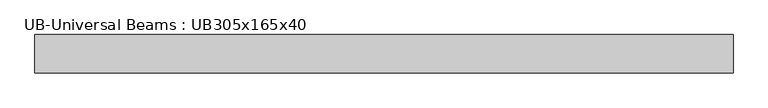
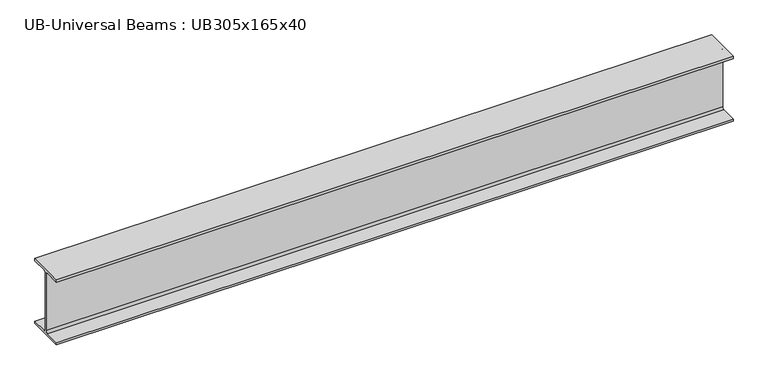
"""IFC4 building model written with IfcOpenShell, lengths in millimetres: beam geometry, UB-Universal Beams : UB305x165x40."""

from ifc_helpers import new_model, si_unit, point, frame, frame_2d, origin, place, context, project, spatial, polyline, circle_curve, trimmed, segment, composite_curve, outline, extrude, source, transform, mapped, element, save


def ub_universal_beams_ub305x165x40_d74fc5b0(model_context):
    return source(origin(), model_context, "Body", "SweptSolid", [
        extrude(outline(composite_curve([segment(polyline([(82.5, -141.5), (82.5, -151.7), (-82.5, -151.7), (-82.5, -141.5), (-11.9, -141.5)]), True, "CONTINUOUS"), segment(trimmed(circle_curve(frame_2d((-11.9, -132.6)), 8.9), [point((-11.9, -141.5))], [point((-3.0, -132.6))], True, "CARTESIAN"), True, "CONTINUOUS"), segment(polyline([(-3.0, -132.6), (-3.0, 132.6)]), True, "CONTINUOUS"), segment(trimmed(circle_curve(frame_2d((-11.9, 132.6)), 8.9), [point((-3.0, 132.6))], [point((-11.9, 141.5))], True, "CARTESIAN"), True, "CONTINUOUS"), segment(polyline([(-11.9, 141.5), (-82.5, 141.5), (-82.5, 151.7), (82.5, 151.7), (82.5, 141.5), (11.9, 141.5)]), True, "CONTINUOUS"), segment(trimmed(circle_curve(frame_2d((11.9, 132.6)), 8.9), [point((11.9, 141.5))], [point((3.0, 132.6))], True, "CARTESIAN"), True, "CONTINUOUS"), segment(polyline([(3.0, 132.6), (3.0, -132.6)]), True, "CONTINUOUS"), segment(trimmed(circle_curve(frame_2d((11.9, -132.6)), 8.9), [point((3.0, -132.6))], [point((11.9, -141.5))], True, "CARTESIAN"), True, "CONTINUOUS"), segment(polyline([(11.9, -141.5), (82.5, -141.5)]), True, "CONTINUOUS")], self_intersect=False)), frame((-1582.5, 0.0, 0.0), z_axis=(1.0, 0.0, 0.0), x_axis=(0.0, 1.0, 0.0)), (0.0, 0.0, 1.0), 2987.3),
    ])


if __name__ == "__main__":
    model = new_model("IFC4")
    model_context = context("Model", 3, world=origin())
    ifc_project = project(units=[si_unit("LENGTHUNIT", "METRE", prefix="MILLI")], contexts=[model_context])
    site = spatial("IfcSite", under=ifc_project)
    building = spatial("IfcBuilding", under=site)
    placement = place(None, origin())
    ub_universal_beams_ub305x165x40_shape = ub_universal_beams_ub305x165x40_d74fc5b0(model_context)
    element("IfcBeam", 1, ObjectType="UB-Universal Beams : UB305x165x40", at=placement, inside=building, context=model_context, shape_type="MappedRepresentation", body=[
        mapped(ub_universal_beams_ub305x165x40_shape, transform((0.0, 0.0, 0.0), x_axis=(1.0, 0.0, 0.0), y_axis=(0.0, 1.0, 0.0), z_axis=(0.0, 0.0, 1.0))),
    ])
    save(model, "model.ifc")

# Revit data of these elements
# Type "UB-Universal Beams : UB305x165x40"
#   Section Name Key = "UB305X165X40"
#   Width = 16.5 cm
#   Web Thickness = 0.6 cm
#   Web Fillet = 0.89 cm
#   Warping Constant = 164000.0 cm⁶
#   Torsional Moment of Inertia = 14.70 cm⁴
#   Section Area = 51.3 cm²
#   Plastic Modulus weak axis = 142.0 cm³
#   Plastic Modulus strong axis = 623.0 cm³
#   Nominal Weight = 40.2999 kgf/m
#   Moment of Inertia weak axis = 764.00 cm⁴
#   Moment of Inertia strong axis = 8503.00 cm⁴
#   Height = 30.34 cm
#   Flange Thickness = 1.02 cm
#   Elastic Modulus weak axis = 92.6 cm³
#   Elastic Modulus strong axis = 560.0 cm³
#   Centroid Vertical = 15.17 cm
#   Centroid Horizontal = 8.25 cm
#   Bolt Spacing = 9.0 cm
#   Length [instance default] = 1.5 m
#   Structural Material [instance default] = Metal - Steel 43-275
#   Type Comments = ""
#   Assembly Code = ""
# Element 1 (IfcBeam, "UB-Universal Beams : UB305x165x40")
#   Materials on its faces: "Metal - Steel 43-275"
# Materials
#   "Metal - Steel 43-275": class "Metal", colour RGB 247 247 247, transparency 0, Cost = 0
